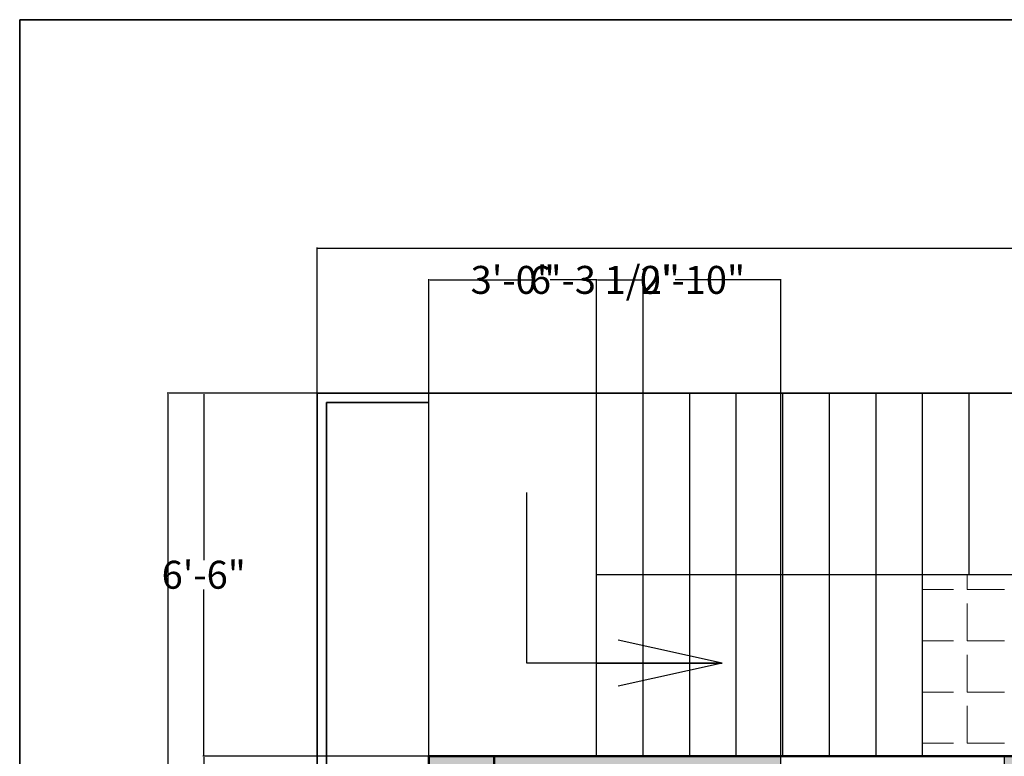
# Model space of a CAD drawing. Units: inches. Extents: x 1601 to 2080, y 5000 to 5589.
# Tile 10 of 11: x 1601 to 1812, y 5431 to 5589. Entities that reach past the tile are written whole.
import ezdxf

# ---------------------------------------------------------------- set-up
doc = ezdxf.new("R2010")
doc.units = ezdxf.units.IN
doc.header["$MEASUREMENT"] = 0
for name, color, linetype, lineweight in [('A-ANNO-DIMS', 2, 'Continuous', 18), ('A-ANNO-TTLB', 7, 'Continuous', 35), ('A-COLS', 7, 'Continuous', 50), ('A-COLS-PATT', 18, 'Continuous', 13), ('A-FLOR-PATT', 8, 'Continuous', 13), ('A-FLOR-STRS', 7, 'Continuous', 25), ('A-GLAZ', 4, 'Continuous', 25), ('A-WALL', 7, 'Continuous', 50), ('A-WALL-PATT', 241, 'Continuous', 13), ('C-PROP', 7, 'Continuous', 35)]:
    doc.layers.add(name, color=color, linetype=linetype, lineweight=lineweight)
doc.styles.get("Standard").update_dxf_attribs({"font": 'arial.ttf'})
doc.dimstyles.get("Standard").update_dxf_attribs({"dimtxt": 6, "dimasz": 0.18, "dimexe": 0.18, "dimexo": 0.0625, "dimgap": 0.09, "dimtad": 0, "dimtih": 1, "dimtoh": 1, "dimdec": 1, "dimzin": 0, "dimdsep": 46, "dimlunit": 3, "dimtxsty": 'Standard', "dimcen": 0.09, "dimadec": 0, "dimazin": 0, "dimtfac": 1, "dimtdec": 1, "dimtofl": 0, "dimtmove": 0, "dimatfit": 3, "dimfxl": 1, "dimtolj": 1, "dimtzin": 0, "dimarcsym": 0})

# ---------------------------------------------------------------- blocks, each defined once
blk = doc.blocks.new('*D3')
at = {"layer": 'A-ANNO-DIMS', "color": 0, "lineweight": -2, "transparency": 16777216}
for p, q in [((1664.41, 5509.26), (1664.41, 5540.54)), ((1664.59, 5540.36), (1838.48, 5540.36)), ((2022.73, 5540.36), (1848.84, 5540.36)), ((2022.91, 5509.26), (2022.91, 5540.54))]:
    blk.add_line(p, q, dxfattribs=at)
at = {"layer": 'A-ANNO-DIMS', "color": 0, "transparency": 16777216}
for points in [[(1664.59, 5540.39), (1664.59, 5540.33), (1664.41, 5540.36)], [(2022.73, 5540.39), (2022.73, 5540.33), (2022.91, 5540.36)]]:
    blk.add_solid(points, dxfattribs=at)
at = {"layer": 'Defpoints', "color": 0, "transparency": 16777216}
for p in [(2022.91, 5540.36), (1664.41, 5509.2), (2022.91, 5509.2)]:
    blk.add_point(p, dxfattribs=at)
at = {"layer": 'A-ANNO-DIMS', "color": 0, "transparency": 16777216, "insert": (1843.66, 5540.36), "char_height": 6, "width": 10.4243, "attachment_point": 5}
blk.add_mtext("\\A1;30'", dxfattribs=at)
blk = doc.blocks.new('*D4')
at = {"layer": 'A-ANNO-DIMS', "color": 0, "lineweight": -2, "transparency": 16777216}
for p, q in [((1664.35, 5509.2), (1632.18, 5509.2)), ((1632.36, 5509.02), (1632.36, 5281.35)), ((1632.36, 5047.39), (1632.36, 5275.05)), ((1664.35, 5047.21), (1632.18, 5047.21))]:
    blk.add_line(p, q, dxfattribs=at)
at = {"layer": 'A-ANNO-DIMS', "color": 0, "transparency": 16777216}
for points in [[(1632.33, 5509.02), (1632.39, 5509.02), (1632.36, 5509.2)], [(1632.33, 5047.39), (1632.39, 5047.39), (1632.36, 5047.21)]]:
    blk.add_solid(points, dxfattribs=at)
at = {"layer": 'Defpoints', "color": 0, "transparency": 16777216}
for p in [(1664.41, 5509.2), (1632.36, 5047.21), (1664.41, 5047.21)]:
    blk.add_point(p, dxfattribs=at)
at = {"layer": 'A-ANNO-DIMS', "color": 0, "transparency": 16777216, "insert": (1632.36, 5278.2), "char_height": 6, "attachment_point": 5}
blk.add_mtext("\\A1;40'", dxfattribs=at)
blk = doc.blocks.new('WINDOW-48IN')
for p, q in [((0, 0), (0, 9)), ((0, 9), (48, 9)), ((48, 9), (48, 0)), ((0, 5.5), (48, 5.5)), ((48, 3.5), (0, 3.5)), ((48, 0), (0, 0))]:
    blk.add_line(p, q)
blk = doc.blocks.new('*D38')
at = {"layer": 'A-ANNO-DIMS', "color": 0, "lineweight": -2, "transparency": 16777216}
for p, q in [((1688.35, 5431.2), (1639.88, 5431.2)), ((1640.06, 5431.02), (1640.06, 5253.64)), ((1640.06, 5069.88), (1640.06, 5247.25)), ((1688.35, 5069.7), (1639.88, 5069.7))]:
    blk.add_line(p, q, dxfattribs=at)
at = {"layer": 'A-ANNO-DIMS', "color": 0, "transparency": 16777216}
for points in [[(1640.03, 5431.02), (1640.09, 5431.02), (1640.06, 5431.2)], [(1640.03, 5069.88), (1640.09, 5069.88), (1640.06, 5069.7)]]:
    blk.add_solid(points, dxfattribs=at)
at = {"layer": 'Defpoints', "color": 0, "transparency": 16777216}
for p in [(1640.06, 5431.2), (1688.41, 5431.2), (1688.41, 5069.7)]:
    blk.add_point(p, dxfattribs=at)
at = {"layer": 'A-ANNO-DIMS', "color": 0, "transparency": 16777216, "insert": (1640.06, 5250.45), "char_height": 6, "attachment_point": 5}
blk.add_mtext('\\A1;30\'-1 1/2"', dxfattribs=at)
blk = doc.blocks.new('*D39')
at = {"layer": 'A-ANNO-DIMS', "color": 0, "lineweight": -2, "transparency": 16777216}
for p, q in [((1688.35, 5509.2), (1639.88, 5509.2)), ((1640.06, 5509.02), (1640.06, 5473.35)), ((1640.06, 5431.38), (1640.06, 5467.04)), ((1688.35, 5431.2), (1639.88, 5431.2))]:
    blk.add_line(p, q, dxfattribs=at)
at = {"layer": 'A-ANNO-DIMS', "color": 0, "transparency": 16777216}
for points in [[(1640.03, 5509.02), (1640.09, 5509.02), (1640.06, 5509.2)], [(1640.03, 5431.38), (1640.09, 5431.38), (1640.06, 5431.2)]]:
    blk.add_solid(points, dxfattribs=at)
at = {"layer": 'Defpoints', "color": 0, "transparency": 16777216}
for p in [(1640.06, 5509.2), (1688.41, 5509.2), (1688.41, 5431.2)]:
    blk.add_point(p, dxfattribs=at)
at = {"layer": 'A-ANNO-DIMS', "color": 0, "transparency": 16777216, "insert": (1640.06, 5470.2), "char_height": 6, "attachment_point": 5}
blk.add_mtext('\\A1;6\'-6"', dxfattribs=at)
blk = doc.blocks.new('*D41')
at = {"layer": 'A-ANNO-DIMS', "color": 0, "lineweight": -2, "transparency": 16777216}
for p, q in [((1688.41, 5509.26), (1688.41, 5533.73)), ((1688.59, 5533.55), (1698.35, 5533.55)), ((1724.23, 5533.55), (1714.47, 5533.55)), ((1724.41, 5509.26), (1724.41, 5533.73))]:
    blk.add_line(p, q, dxfattribs=at)
at = {"layer": 'A-ANNO-DIMS', "color": 0, "transparency": 16777216}
for points in [[(1688.59, 5533.58), (1688.59, 5533.52), (1688.41, 5533.55)], [(1724.23, 5533.58), (1724.23, 5533.52), (1724.41, 5533.55)]]:
    blk.add_solid(points, dxfattribs=at)
at = {"layer": 'Defpoints', "color": 0, "transparency": 16777216}
for p in [(1724.41, 5533.55), (1688.41, 5509.2), (1724.41, 5509.2)]:
    blk.add_point(p, dxfattribs=at)
at = {"layer": 'A-ANNO-DIMS', "color": 0, "transparency": 16777216, "insert": (1706.41, 5533.55), "char_height": 6, "attachment_point": 5}
blk.add_mtext('\\A1;3\'-0"', dxfattribs=at)
blk = doc.blocks.new('*D42')
at = {"layer": 'A-ANNO-DIMS', "color": 0, "lineweight": -2, "transparency": 16777216}
for p, q in [((1724.41, 5509.26), (1724.41, 5533.73)), ((1724.59, 5533.55), (1734.23, 5533.55)), ((1734.41, 5509.26), (1734.41, 5533.73)), ((1734.41, 5533.55), (1734.59, 5533.55))]:
    blk.add_line(p, q, dxfattribs=at)
at = {"layer": 'A-ANNO-DIMS', "color": 0, "transparency": 16777216}
for points in [[(1724.59, 5533.58), (1724.59, 5533.52), (1724.41, 5533.55)], [(1734.23, 5533.58), (1734.23, 5533.52), (1734.41, 5533.55)]]:
    blk.add_solid(points, dxfattribs=at)
at = {"layer": 'Defpoints', "color": 0, "transparency": 16777216}
for p in [(1734.41, 5533.55), (1724.41, 5509.2), (1734.41, 5509.2)]:
    blk.add_point(p, dxfattribs=at)
at = {"layer": 'A-ANNO-DIMS', "color": 0, "transparency": 16777216, "insert": (1744.98, 5533.55), "char_height": 6, "attachment_point": 5}
blk.add_mtext('\\A1;0\'-10"', dxfattribs=at)
blk = doc.blocks.new('*D47')
at = {"layer": 'A-ANNO-DIMS', "color": 0, "lineweight": -2, "transparency": 16777216}
for p, q in [((1688.41, 5431.26), (1688.41, 5533.73)), ((1688.59, 5533.55), (1711.11, 5533.55)), ((1763.77, 5533.55), (1741.25, 5533.55)), ((1763.95, 5431.26), (1763.95, 5533.73))]:
    blk.add_line(p, q, dxfattribs=at)
at = {"layer": 'A-ANNO-DIMS', "color": 0, "transparency": 16777216}
for points in [[(1688.59, 5533.58), (1688.59, 5533.52), (1688.41, 5533.55)], [(1763.77, 5533.58), (1763.77, 5533.52), (1763.95, 5533.55)]]:
    blk.add_solid(points, dxfattribs=at)
at = {"layer": 'Defpoints', "color": 0, "transparency": 16777216}
for p in [(1763.95, 5533.55), (1688.41, 5431.2), (1763.95, 5431.2)]:
    blk.add_point(p, dxfattribs=at)
at = {"layer": 'A-ANNO-DIMS', "color": 0, "transparency": 16777216, "insert": (1726.18, 5533.55), "char_height": 6, "attachment_point": 5}
blk.add_mtext('\\A1;6\'-3 1/2"', dxfattribs=at)

msp = doc.modelspace()

# ---------------------------------------------------------------- hatches: boundary and pattern name
at = {"layer": 'A-COLS-PATT'}
h = msp.add_hatch(color=256, dxfattribs=at)
h.dxf.hatch_style = 1
h.paths.add_polyline_path([(1702.41, 5431.2), (1688.41, 5431.2), (1688.41, 5422.2), (1702.41, 5422.2)])
h.paths.add_polyline_path([(1836.17, 5431.2), (1822.17, 5431.2), (1822.17, 5422.2), (1836.17, 5422.2)])
h.paths.add_polyline_path([(1962.91, 5431.2), (1948.91, 5431.2), (1948.91, 5422.2), (1962.91, 5422.2)])
h.paths.add_polyline_path([(1697.41, 5314.2), (1688.41, 5314.2), (1688.41, 5300.2), (1697.41, 5300.2)])
h.paths.add_polyline_path([(1833.91, 5314.2), (1824.91, 5314.2), (1824.91, 5300.2), (1833.91, 5300.2)])
h.paths.add_polyline_path([(1962.91, 5314.2), (1953.91, 5314.2), (1953.91, 5300.2), (1962.91, 5300.2)])
h.paths.add_polyline_path([(1697.41, 5209.2), (1688.41, 5209.2), (1688.41, 5195.2), (1697.41, 5195.2)])
h.paths.add_polyline_path([(1833.91, 5209.2), (1824.91, 5209.2), (1824.91, 5195.2), (1833.91, 5195.2)])
h.paths.add_polyline_path([(1962.91, 5209.2), (1953.91, 5209.2), (1953.91, 5195.2), (1962.91, 5195.2)])
h.paths.add_polyline_path([(1697.41, 5083.7), (1688.41, 5083.7), (1688.41, 5069.7), (1697.41, 5069.7)])
h.paths.add_polyline_path([(1833.91, 5078.7), (1819.91, 5078.7), (1819.91, 5069.7), (1833.91, 5069.7)])
h.paths.add_polyline_path([(1962.91, 5078.7), (1948.91, 5078.7), (1948.91, 5069.7), (1962.91, 5069.7)])
at = {"layer": 'A-FLOR-PATT'}
h = msp.add_hatch(dxfattribs=at)
h.set_pattern_fill('ANGLE', color=256, scale=40)
h.set_pattern_definition([(0, (0, 0), (0, 11), [8, -3]), (90, (0, 0), (-11, 7e-16), [8, -3])])
h.paths.add_polyline_path([(2022.91, 5509.2), (1941.91, 5509.2), (1911.91, 5509.2), (1864.41, 5509.2), (1864.41, 5489.7), (1868.54, 5489.7, -0.022155), (1868.52, 5490.01, -1), (1875.53, 5490.01, -0.956651), (1868.54, 5489.7), (1864.41, 5489.7), (1864.41, 5470.2), (1794.41, 5470.2), (1794.41, 5431.2), (1811.95, 5431.2), (1911.91, 5431.2), (1941.91, 5431.2), (1942.91, 5431.2), (1945.91, 5431.2), (1948.91, 5431.2), (1962.91, 5431.2), (1962.91, 5415.29), (1962.91, 5385.29), (1962.91, 5384.29), (1962.91, 5381.29), (1962.91, 5333.29), (1962.91, 5069.7), (2022.91, 5069.7)])
h.paths.add_polyline_path([(2000.28, 5267.55), (2000.28, 5367.64), (1987.91, 5367.64), (1987.91, 5267.55)], flags=24)
h.paths.add_polyline_path([(1879.42, 5455.52), (1969.04, 5455.52), (1969.04, 5467.88), (1879.42, 5467.88)], flags=24)
at = {"layer": 'A-WALL-PATT'}
h = msp.add_hatch(color=256, dxfattribs=at)
h.dxf.hatch_style = 1
h.paths.add_polyline_path([(1763.95, 5431.2), (1702.41, 5431.2), (1702.41, 5422.2), (1763.95, 5422.2)])
h.paths.add_polyline_path([(1697.41, 5422.2), (1688.41, 5422.2), (1688.41, 5314.2), (1697.41, 5314.2)])
h.paths.add_polyline_path([(1740.41, 5314.2), (1697.41, 5314.2), (1697.41, 5309.7), (1740.41, 5309.7)], flags=17)
h.paths.add_polyline_path([(1822.17, 5431.2), (1811.95, 5431.2), (1811.95, 5422.2), (1822.17, 5422.2)])
h.paths.add_polyline_path([(1845.52, 5431.2), (1836.17, 5431.2), (1836.17, 5422.2), (1845.52, 5422.2)])
h.paths.add_polyline_path([(1910.91, 5431.2), (1881.52, 5431.2), (1881.52, 5422.2), (1910.91, 5422.2)])
h.paths.add_polyline_path([(1948.91, 5431.2), (1945.91, 5431.2), (1942.91, 5431.2), (1942.91, 5422.2), (1948.91, 5422.2)])
h.paths.add_polyline_path([(1962.91, 5422.2), (1953.91, 5422.2), (1953.91, 5416.29), (1962.91, 5416.29)])
h.paths.add_polyline_path([(1962.91, 5384.29), (1953.91, 5384.29), (1953.91, 5381.29), (1962.91, 5381.29)])
h.paths.add_polyline_path([(1962.91, 5333.29), (1953.91, 5333.29), (1953.91, 5314.2), (1962.91, 5314.2)])
h.paths.add_polyline_path([(1962.91, 5300.2), (1953.91, 5300.2), (1953.91, 5236.2), (1875.91, 5236.2), (1875.91, 5230.7), (1881.91, 5230.7), (1881.91, 5231.7), (1953.91, 5231.7), (1953.91, 5219.2), (1962.91, 5219.2)])
h.paths.add_polyline_path([(1962.91, 5185.2), (1953.91, 5185.2), (1953.91, 5183.7), (1881.91, 5183.7), (1881.91, 5184.7), (1875.91, 5184.7), (1875.91, 5183.7), (1875.91, 5179.2), (1953.91, 5179.2), (1953.91, 5172.6), (1962.91, 5172.6)])
h.paths.add_polyline_path([(1962.91, 5136.6), (1953.91, 5136.6), (1953.91, 5078.7), (1962.91, 5078.7)])
h.paths.add_polyline_path([(1948.91, 5078.7), (1833.91, 5078.7), (1833.91, 5069.7), (1948.91, 5069.7)])
h.paths.add_polyline_path([(1833.91, 5195.2), (1829.41, 5195.2), (1829.41, 5078.7), (1833.91, 5078.7)])
h.paths.add_polyline_path([(1819.91, 5078.7), (1813.58, 5078.7), (1813.58, 5069.7), (1819.91, 5069.7)])
h.paths.add_polyline_path([(1765.58, 5078.7), (1697.41, 5078.7), (1697.41, 5069.7), (1765.58, 5069.7)])
h.paths.add_polyline_path([(1697.41, 5195.2), (1688.41, 5195.2), (1688.41, 5083.7), (1697.41, 5083.7)])
h.paths.add_polyline_path([(1740.41, 5209.2), (1697.41, 5209.2), (1697.41, 5204.7), (1740.41, 5204.7)], flags=17)
h.paths.add_polyline_path([(1787.91, 5209.2), (1779.91, 5209.2), (1779.91, 5309.7), (1787.91, 5309.7), (1787.91, 5314.2), (1772.41, 5314.2), (1772.41, 5309.7), (1775.41, 5309.7), (1775.41, 5261.7), (1697.41, 5261.7), (1697.41, 5273.07), (1688.41, 5273.07), (1688.41, 5242.37), (1697.41, 5242.37), (1697.41, 5257.2), (1775.41, 5257.2), (1775.41, 5209.2), (1772.41, 5209.2), (1772.41, 5204.7), (1775.41, 5204.7), (1787.91, 5204.7)])
h.paths.add_polyline_path([(1697.41, 5218.37), (1688.41, 5218.37), (1688.41, 5209.2), (1697.41, 5209.2)], flags=17)
h.paths.add_polyline_path([(1833.91, 5422.2), (1829.41, 5422.2), (1829.41, 5314.2), (1833.91, 5314.2)])
h.paths.add_polyline_path([(1697.41, 5300.2), (1688.41, 5300.2), (1688.41, 5297.07), (1697.41, 5297.07)], flags=17)

# ---------------------------------------------------------------- linework, layer by layer
at = {"layer": 'A-ANNO-TTLB'}
msp.add_lwpolyline([(1600.55, 5589.45), (2079.72, 5589.45), (2079.72, 4999.95), (1600.55, 4999.95)], close=True, dxfattribs=at)
at = {"layer": 'A-COLS'}
msp.add_line((1702.41, 5431.2), (1702.41, 5422.2), dxfattribs=at)
at = {"layer": 'A-FLOR-STRS'}
for p, q in [((1688.41, 5431.2), (1688.41, 5509.2)), ((1724.41, 5431.2), (1724.41, 5509.2)), ((1734.41, 5431.2), (1734.41, 5509.2)), ((1744.41, 5431.2), (1744.41, 5509.2)), ((1754.41, 5431.2), (1754.41, 5509.2)), ((1764.41, 5431.2), (1764.41, 5509.2)), ((1774.41, 5431.2), (1774.41, 5509.2)), ((1784.41, 5431.2), (1784.41, 5509.2)), ((1794.41, 5431.2), (1794.41, 5509.2)), ((1804.41, 5470.2), (1804.41, 5509.2)), ((1709.41, 5451.23), (1709.41, 5487.89)), ((1864.41, 5470.2), (1724.41, 5470.2)), ((1751.37, 5451.23), (1729.03, 5456.18)), ((1751.37, 5451.23), (1709.41, 5451.23)), ((1724.41, 5451.23), (1751.37, 5451.23)), ((1751.37, 5451.23), (1729.03, 5446.28))]:
    msp.add_line(p, q, dxfattribs=at)
at = {"layer": 'A-WALL'}
for q in [(1911.91, 5431.2), (1688.41, 5069.7)]:
    msp.add_line((1688.41, 5431.2), q, dxfattribs=at)
at = {"layer": 'C-PROP'}
for p, q in [((1664.41, 5509.2), (1664.41, 5047.21)), ((1664.41, 5509.2), (1911.91, 5509.2)), ((1666.41, 5507.2), (1688.41, 5507.2)), ((1666.41, 5507.2), (1666.41, 5069.7))]:
    msp.add_line(p, q, dxfattribs=at)

# ---------------------------------------------------------------- block references
at = {"layer": 'A-GLAZ'}
msp.add_blockref('WINDOW-48IN', (1763.95, 5422.2), dxfattribs=at)

# ---------------------------------------------------------------- dimensions: what is measured, and where the dimension line sits
at = {"layer": 'A-ANNO-DIMS'}
dim = msp.add_linear_dim(base=(2022.91, 5540.36), p1=(1664.41, 5509.2), p2=(2022.91, 5509.2), text="30'", dimstyle='Standard', override={"dimclrd": 0, "dimclre": 0, "dimclrt": 0}, dxfattribs=at)
dim.commit()
dim.dimension.update_dxf_attribs({"geometry": '*D3', "text_midpoint": (1843.66, 5540.36)})
for base, p1, p2, picture, middle in [((1763.95, 5533.55), (1688.41, 5431.2), (1763.95, 5431.2), '*D47', (1726.18, 5533.55)), ((1724.41, 5533.55), (1688.41, 5509.2), (1724.41, 5509.2), '*D41', (1706.41, 5533.55)), ((1734.41, 5533.55), (1724.41, 5509.2), (1734.41, 5509.2), '*D42', (1744.98, 5533.55))]:
    dim = msp.add_linear_dim(base=base, p1=p1, p2=p2, dimstyle='Standard', override={"dimdec": 1, "dimlfac": 1, "dimrnd": 0, "dimzin": 1, "dimdsep": 46, "dimlunit": 4, "dimfrac": 2}, dxfattribs=at)
    dim.commit()
    dim.dimension.update_dxf_attribs({"geometry": picture, "text_midpoint": middle})
dim = msp.add_linear_dim(base=(1632.36, 5047.21), p1=(1664.41, 5509.2), p2=(1664.41, 5047.21), angle=90, text="40'", dimstyle='Standard', override={"dimclrd": 0, "dimclre": 0, "dimclrt": 0}, dxfattribs=at)
dim.commit()
dim.dimension.update_dxf_attribs({"geometry": '*D4', "text_midpoint": (1632.36, 5278.2)})
for base, p1, p2, picture, middle in [((1640.06, 5509.2), (1688.41, 5431.2), (1688.41, 5509.2), '*D39', (1640.06, 5470.2)), ((1640.06, 5431.2), (1688.41, 5069.7), (1688.41, 5431.2), '*D38', (1640.06, 5250.45))]:
    dim = msp.add_linear_dim(base=base, p1=p1, p2=p2, angle=90, dimstyle='Standard', override={"dimdec": 1, "dimlfac": 1, "dimrnd": 0, "dimzin": 1, "dimdsep": 46, "dimlunit": 4, "dimfrac": 2}, dxfattribs=at)
    dim.commit()
    dim.dimension.update_dxf_attribs({"geometry": picture, "text_midpoint": middle})

doc.saveas('drawing.dxf')
